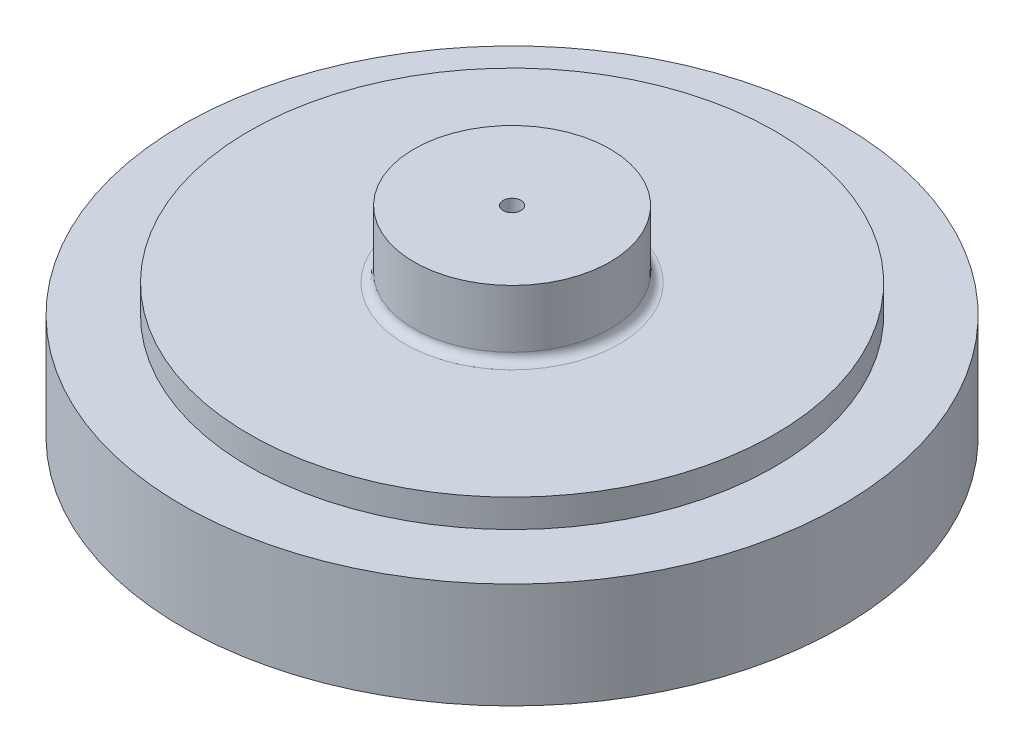
ISO-10303-21;
HEADER;
FILE_DESCRIPTION(('STEP AP214'),'2;1');
FILE_NAME('part.step','',(''),(''),'','','');
FILE_SCHEMA(('AUTOMOTIVE_DESIGN { 1 0 10303 214 1 1 1 1 }'));
ENDSEC;
DATA;
#1=APPLICATION_CONTEXT('core data for automotive mechanical design processes');
#2=APPLICATION_PROTOCOL_DEFINITION('international standard','automotive_design',2000,#1);
#3=PRODUCT_CONTEXT('',#1,'mechanical');
#4=PRODUCT('Part','Part','',(#3));
#5=PRODUCT_RELATED_PRODUCT_CATEGORY('part','',(#4));
#6=PRODUCT_DEFINITION_FORMATION('','',#4);
#7=PRODUCT_DEFINITION_CONTEXT('part definition',#1,'design');
#8=PRODUCT_DEFINITION('design','',#6,#7);
#9=PRODUCT_DEFINITION_SHAPE('','',#8);
#10=(LENGTH_UNIT() NAMED_UNIT(*) SI_UNIT(.MILLI.,.METRE.));
#11=(NAMED_UNIT(*) PLANE_ANGLE_UNIT() SI_UNIT($,.RADIAN.));
#12=(NAMED_UNIT(*) SI_UNIT($,.STERADIAN.) SOLID_ANGLE_UNIT());
#13=UNCERTAINTY_MEASURE_WITH_UNIT(LENGTH_MEASURE(1.E-05),#10,'distance_accuracy_value','');
#14=(GEOMETRIC_REPRESENTATION_CONTEXT(3) GLOBAL_UNCERTAINTY_ASSIGNED_CONTEXT((#13)) GLOBAL_UNIT_ASSIGNED_CONTEXT((#10,
#11,#12)) REPRESENTATION_CONTEXT('',''));
#15=CARTESIAN_POINT('',(0.,0.,0.));
#16=DIRECTION('',(0.,0.,1.));
#17=DIRECTION('',(1.,0.,0.));
#18=AXIS2_PLACEMENT_3D('',#15,#16,#17);
#19=CARTESIAN_POINT('',(0.,0.,0.));
#20=DIRECTION('',(0.,-1.,0.));
#21=DIRECTION('',(0.,0.,-1.));
#22=AXIS2_PLACEMENT_3D('',#19,#20,#21);
#23=PLANE('',#22);
#24=CARTESIAN_POINT('',(-45.,0.,0.));
#25=DIRECTION('',(0.,1.,0.));
#26=DIRECTION('',(0.,0.,1.));
#27=AXIS2_PLACEMENT_3D('',#24,#25,#26);
#28=CIRCLE('',#27,6.);
#29=CARTESIAN_POINT('',(-45.,0.,6.));
#30=VERTEX_POINT('',#29);
#31=EDGE_CURVE('E72',#30,#30,#28,.T.);
#32=ORIENTED_EDGE('',*,*,#31,.T.);
#33=EDGE_LOOP('',(#32));
#34=FACE_BOUND('',#33,.T.);
#35=CARTESIAN_POINT('',(45.,0.,0.));
#36=DIRECTION('',(0.,1.,0.));
#37=DIRECTION('',(0.,0.,1.));
#38=AXIS2_PLACEMENT_3D('',#35,#36,#37);
#39=CIRCLE('',#38,6.);
#40=CARTESIAN_POINT('',(45.,0.,6.));
#41=VERTEX_POINT('',#40);
#42=EDGE_CURVE('E73',#41,#41,#39,.T.);
#43=ORIENTED_EDGE('',*,*,#42,.T.);
#44=EDGE_LOOP('',(#43));
#45=FACE_BOUND('',#44,.T.);
#46=CARTESIAN_POINT('',(0.,0.,0.));
#47=DIRECTION('',(0.,-1.,0.));
#48=DIRECTION('',(0.,0.,-1.));
#49=AXIS2_PLACEMENT_3D('',#46,#47,#48);
#50=CIRCLE('',#49,74.);
#51=CARTESIAN_POINT('',(0.,0.,-74.));
#52=VERTEX_POINT('',#51);
#53=EDGE_CURVE('E68',#52,#52,#50,.T.);
#54=ORIENTED_EDGE('',*,*,#53,.T.);
#55=EDGE_LOOP('',(#54));
#56=FACE_BOUND('',#55,.T.);
#57=ADVANCED_FACE('F40',(#34,#45,#56),#23,.T.);
#58=CARTESIAN_POINT('',(0.,30.,0.));
#59=DIRECTION('',(0.,1.,0.));
#60=DIRECTION('',(0.,0.,1.));
#61=AXIS2_PLACEMENT_3D('',#58,#59,#60);
#62=PLANE('',#61);
#63=CARTESIAN_POINT('',(0.,30.,0.));
#64=DIRECTION('',(0.,-1.,0.));
#65=DIRECTION('',(0.,0.,-1.));
#66=AXIS2_PLACEMENT_3D('',#63,#64,#65);
#67=CIRCLE('',#66,2.);
#68=CARTESIAN_POINT('',(0.,30.,-2.));
#69=VERTEX_POINT('',#68);
#70=EDGE_CURVE('E10',#69,#69,#67,.T.);
#71=ORIENTED_EDGE('',*,*,#70,.F.);
#72=EDGE_LOOP('',(#71));
#73=FACE_BOUND('',#72,.T.);
#74=ADVANCED_FACE('F97',(#73),#62,.T.);
#75=CARTESIAN_POINT('',(0.,0.,0.));
#76=DIRECTION('',(0.,-1.,0.));
#77=DIRECTION('',(0.,0.,-1.));
#78=AXIS2_PLACEMENT_3D('',#75,#76,#77);
#79=CYLINDRICAL_SURFACE('',#78,2.);
#80=ORIENTED_EDGE('',*,*,#70,.T.);
#81=EDGE_LOOP('',(#80));
#82=FACE_BOUND('',#81,.T.);
#83=CARTESIAN_POINT('',(0.,45.,0.));
#84=DIRECTION('',(0.,-1.,0.));
#85=DIRECTION('',(0.,0.,-1.));
#86=AXIS2_PLACEMENT_3D('',#83,#84,#85);
#87=CIRCLE('',#86,2.);
#88=CARTESIAN_POINT('',(0.,45.,-2.));
#89=VERTEX_POINT('',#88);
#90=EDGE_CURVE('E43',#89,#89,#87,.T.);
#91=ORIENTED_EDGE('',*,*,#90,.F.);
#92=EDGE_LOOP('',(#91));
#93=FACE_BOUND('',#92,.T.);
#94=ADVANCED_FACE('F104',(#82,#93),#79,.F.);
#95=CARTESIAN_POINT('',(2.,45.,0.));
#96=DIRECTION('',(0.,1.,0.));
#97=DIRECTION('',(0.,0.,1.));
#98=AXIS2_PLACEMENT_3D('',#95,#96,#97);
#99=PLANE('',#98);
#100=ORIENTED_EDGE('',*,*,#90,.T.);
#101=EDGE_LOOP('',(#100));
#102=FACE_BOUND('',#101,.T.);
#103=CARTESIAN_POINT('',(0.,45.,0.));
#104=DIRECTION('',(0.,-1.,0.));
#105=DIRECTION('',(0.,0.,-1.));
#106=AXIS2_PLACEMENT_3D('',#103,#104,#105);
#107=CIRCLE('',#106,22.);
#108=CARTESIAN_POINT('',(0.,45.,-22.));
#109=VERTEX_POINT('',#108);
#110=EDGE_CURVE('E50',#109,#109,#107,.T.);
#111=ORIENTED_EDGE('',*,*,#110,.F.);
#112=EDGE_LOOP('',(#111));
#113=FACE_BOUND('',#112,.T.);
#114=ADVANCED_FACE('F109',(#102,#113),#99,.T.);
#115=CARTESIAN_POINT('',(0.,0.,0.));
#116=DIRECTION('',(0.,-1.,0.));
#117=DIRECTION('',(0.,0.,-1.));
#118=AXIS2_PLACEMENT_3D('',#115,#116,#117);
#119=CYLINDRICAL_SURFACE('',#118,22.);
#120=ORIENTED_EDGE('',*,*,#110,.T.);
#121=EDGE_LOOP('',(#120));
#122=FACE_BOUND('',#121,.T.);
#123=CARTESIAN_POINT('',(0.,32.,0.));
#124=DIRECTION('',(0.,-1.,0.));
#125=DIRECTION('',(0.,0.,-1.));
#126=AXIS2_PLACEMENT_3D('',#123,#124,#125);
#127=CIRCLE('',#126,22.);
#128=CARTESIAN_POINT('',(0.,32.,-22.));
#129=VERTEX_POINT('',#128);
#130=EDGE_CURVE('E51',#129,#129,#127,.T.);
#131=ORIENTED_EDGE('',*,*,#130,.F.);
#132=EDGE_LOOP('',(#131));
#133=FACE_BOUND('',#132,.T.);
#134=ADVANCED_FACE('F113',(#122,#133),#119,.T.);
#135=CARTESIAN_POINT('',(0.,32.,0.));
#136=DIRECTION('',(0.,-1.,0.));
#137=DIRECTION('',(0.,0.,-1.));
#138=AXIS2_PLACEMENT_3D('',#135,#136,#137);
#139=TOROIDAL_SURFACE('',#138,24.,2.);
#140=ORIENTED_EDGE('',*,*,#130,.T.);
#141=EDGE_LOOP('',(#140));
#142=FACE_BOUND('',#141,.T.);
#143=CARTESIAN_POINT('',(0.,30.,0.));
#144=DIRECTION('',(0.,-1.,0.));
#145=DIRECTION('',(0.,0.,-1.));
#146=AXIS2_PLACEMENT_3D('',#143,#144,#145);
#147=CIRCLE('',#146,24.);
#148=CARTESIAN_POINT('',(0.,30.,-24.));
#149=VERTEX_POINT('',#148);
#150=EDGE_CURVE('E57',#149,#149,#147,.T.);
#151=ORIENTED_EDGE('',*,*,#150,.F.);
#152=EDGE_LOOP('',(#151));
#153=FACE_BOUND('',#152,.T.);
#154=ADVANCED_FACE('F117',(#142,#153),#139,.F.);
#155=CARTESIAN_POINT('',(24.,30.,0.));
#156=DIRECTION('',(0.,1.,0.));
#157=DIRECTION('',(0.,0.,1.));
#158=AXIS2_PLACEMENT_3D('',#155,#156,#157);
#159=PLANE('',#158);
#160=ORIENTED_EDGE('',*,*,#150,.T.);
#161=EDGE_LOOP('',(#160));
#162=FACE_BOUND('',#161,.T.);
#163=CARTESIAN_POINT('',(0.,30.,0.));
#164=DIRECTION('',(0.,-1.,0.));
#165=DIRECTION('',(0.,0.,-1.));
#166=AXIS2_PLACEMENT_3D('',#163,#164,#165);
#167=CIRCLE('',#166,59.);
#168=CARTESIAN_POINT('',(0.,30.,-59.));
#169=VERTEX_POINT('',#168);
#170=EDGE_CURVE('E56',#169,#169,#167,.T.);
#171=ORIENTED_EDGE('',*,*,#170,.F.);
#172=EDGE_LOOP('',(#171));
#173=FACE_BOUND('',#172,.T.);
#174=ADVANCED_FACE('F125',(#162,#173),#159,.T.);
#175=CARTESIAN_POINT('',(0.,0.,0.));
#176=DIRECTION('',(0.,-1.,0.));
#177=DIRECTION('',(0.,0.,-1.));
#178=AXIS2_PLACEMENT_3D('',#175,#176,#177);
#179=CYLINDRICAL_SURFACE('',#178,59.);
#180=ORIENTED_EDGE('',*,*,#170,.T.);
#181=EDGE_LOOP('',(#180));
#182=FACE_BOUND('',#181,.T.);
#183=CARTESIAN_POINT('',(0.,23.7,0.));
#184=DIRECTION('',(0.,-1.,0.));
#185=DIRECTION('',(0.,0.,-1.));
#186=AXIS2_PLACEMENT_3D('',#183,#184,#185);
#187=CIRCLE('',#186,59.);
#188=CARTESIAN_POINT('',(0.,23.7,-59.));
#189=VERTEX_POINT('',#188);
#190=EDGE_CURVE('E64',#189,#189,#187,.T.);
#191=ORIENTED_EDGE('',*,*,#190,.F.);
#192=EDGE_LOOP('',(#191));
#193=FACE_BOUND('',#192,.T.);
#194=ADVANCED_FACE('F127',(#182,#193),#179,.T.);
#195=CARTESIAN_POINT('',(59.,23.7,0.));
#196=DIRECTION('',(0.,1.,0.));
#197=DIRECTION('',(0.,0.,1.));
#198=AXIS2_PLACEMENT_3D('',#195,#196,#197);
#199=PLANE('',#198);
#200=ORIENTED_EDGE('',*,*,#190,.T.);
#201=EDGE_LOOP('',(#200));
#202=FACE_BOUND('',#201,.T.);
#203=CARTESIAN_POINT('',(0.,23.7,0.));
#204=DIRECTION('',(0.,-1.,0.));
#205=DIRECTION('',(0.,0.,-1.));
#206=AXIS2_PLACEMENT_3D('',#203,#204,#205);
#207=CIRCLE('',#206,74.);
#208=CARTESIAN_POINT('',(0.,23.7,-74.));
#209=VERTEX_POINT('',#208);
#210=EDGE_CURVE('E61',#209,#209,#207,.T.);
#211=ORIENTED_EDGE('',*,*,#210,.F.);
#212=EDGE_LOOP('',(#211));
#213=FACE_BOUND('',#212,.T.);
#214=ADVANCED_FACE('F128',(#202,#213),#199,.T.);
#215=CARTESIAN_POINT('',(0.,0.,0.));
#216=DIRECTION('',(0.,-1.,0.));
#217=DIRECTION('',(0.,0.,-1.));
#218=AXIS2_PLACEMENT_3D('',#215,#216,#217);
#219=CYLINDRICAL_SURFACE('',#218,74.);
#220=ORIENTED_EDGE('',*,*,#210,.T.);
#221=EDGE_LOOP('',(#220));
#222=FACE_BOUND('',#221,.T.);
#223=ORIENTED_EDGE('',*,*,#53,.F.);
#224=EDGE_LOOP('',(#223));
#225=FACE_BOUND('',#224,.T.);
#226=ADVANCED_FACE('F135',(#222,#225),#219,.T.);
#227=CARTESIAN_POINT('',(45.,0.,0.));
#228=DIRECTION('',(0.,1.,0.));
#229=DIRECTION('',(0.,0.,1.));
#230=AXIS2_PLACEMENT_3D('',#227,#228,#229);
#231=CYLINDRICAL_SURFACE('',#230,6.);
#232=ORIENTED_EDGE('',*,*,#42,.F.);
#233=EDGE_LOOP('',(#232));
#234=FACE_BOUND('',#233,.T.);
#235=CARTESIAN_POINT('',(45.,23.7,0.));
#236=DIRECTION('',(0.,1.,0.));
#237=DIRECTION('',(0.,0.,1.));
#238=AXIS2_PLACEMENT_3D('',#235,#236,#237);
#239=CIRCLE('',#238,6.);
#240=CARTESIAN_POINT('',(45.,23.7,6.));
#241=VERTEX_POINT('',#240);
#242=EDGE_CURVE('E75',#241,#241,#239,.T.);
#243=ORIENTED_EDGE('',*,*,#242,.T.);
#244=EDGE_LOOP('',(#243));
#245=FACE_BOUND('',#244,.T.);
#246=ADVANCED_FACE('F140',(#234,#245),#231,.F.);
#247=CARTESIAN_POINT('',(45.,23.7,0.));
#248=DIRECTION('',(0.,1.,0.));
#249=DIRECTION('',(0.,0.,1.));
#250=AXIS2_PLACEMENT_3D('',#247,#248,#249);
#251=PLANE('',#250);
#252=ORIENTED_EDGE('',*,*,#242,.F.);
#253=EDGE_LOOP('',(#252));
#254=FACE_BOUND('',#253,.T.);
#255=ADVANCED_FACE('F89',(#254),#251,.F.);
#256=CARTESIAN_POINT('',(-45.,0.,0.));
#257=DIRECTION('',(0.,1.,0.));
#258=DIRECTION('',(0.,0.,1.));
#259=AXIS2_PLACEMENT_3D('',#256,#257,#258);
#260=CYLINDRICAL_SURFACE('',#259,6.);
#261=ORIENTED_EDGE('',*,*,#31,.F.);
#262=EDGE_LOOP('',(#261));
#263=FACE_BOUND('',#262,.T.);
#264=CARTESIAN_POINT('',(-45.,23.7,0.));
#265=DIRECTION('',(0.,1.,0.));
#266=DIRECTION('',(0.,0.,1.));
#267=AXIS2_PLACEMENT_3D('',#264,#265,#266);
#268=CIRCLE('',#267,6.);
#269=CARTESIAN_POINT('',(-45.,23.7,6.));
#270=VERTEX_POINT('',#269);
#271=EDGE_CURVE('E77',#270,#270,#268,.T.);
#272=ORIENTED_EDGE('',*,*,#271,.T.);
#273=EDGE_LOOP('',(#272));
#274=FACE_BOUND('',#273,.T.);
#275=ADVANCED_FACE('F88',(#263,#274),#260,.F.);
#276=CARTESIAN_POINT('',(-45.,23.7,0.));
#277=DIRECTION('',(0.,1.,0.));
#278=DIRECTION('',(0.,0.,1.));
#279=AXIS2_PLACEMENT_3D('',#276,#277,#278);
#280=PLANE('',#279);
#281=ORIENTED_EDGE('',*,*,#271,.F.);
#282=EDGE_LOOP('',(#281));
#283=FACE_BOUND('',#282,.T.);
#284=ADVANCED_FACE('F90',(#283),#280,.F.);
#285=CLOSED_SHELL('',(#57,#74,#94,#114,#134,#154,#174,#194,#214,#226,#246,#255,#275,#284));
#286=MANIFOLD_SOLID_BREP('B2',#285);
#287=ADVANCED_BREP_SHAPE_REPRESENTATION('',(#18,#286),#14);
#288=SHAPE_DEFINITION_REPRESENTATION(#9,#287);
ENDSEC;
END-ISO-10303-21;
